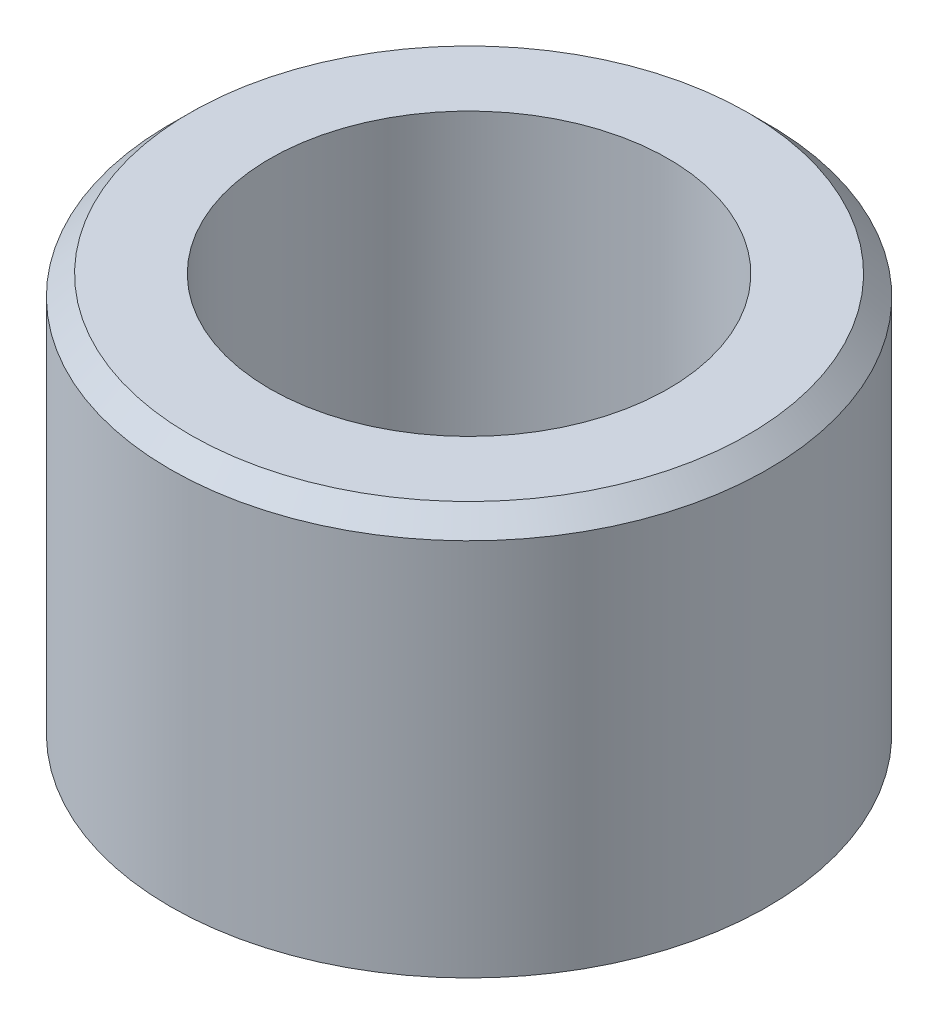
from build123d import *

# Parameters (mm, degrees)
BUSH_PROFILE_30_20_R         = 15
BUSH_PROFILE_30_20_R_2       = 10
BUSH_BODY_L20_DEPTH          = 20
OUTER_EDGE_CHAMFER_1X45_SIZE = 1


with BuildPart() as part:
    # Bush Profile Ø30-Ø20 → Bush Body L20 (new body)
    with BuildSketch(Plane(origin=(0, 0, 0), x_dir=(1, 0, 0), z_dir=(0, 1, 0))):
        with Locations(Location((0, 0, 0), (0, 0, 270))):
            Circle(BUSH_PROFILE_30_20_R)
        with Locations(Location((0, 0, 0), (0, 0, 270))):
            Circle(BUSH_PROFILE_30_20_R_2, mode=Mode.SUBTRACT)
    extrude(amount=BUSH_BODY_L20_DEPTH)

    # Outer Edge Chamfer 1x45°
    outer_edge_chamfer_1x45_edges = [part.edges().sort_by_distance(p)[0] for p in [
        (0, 20, -15),
    ]]
    chamfer(outer_edge_chamfer_1x45_edges, length=OUTER_EDGE_CHAMFER_1X45_SIZE)


solid = part.part
